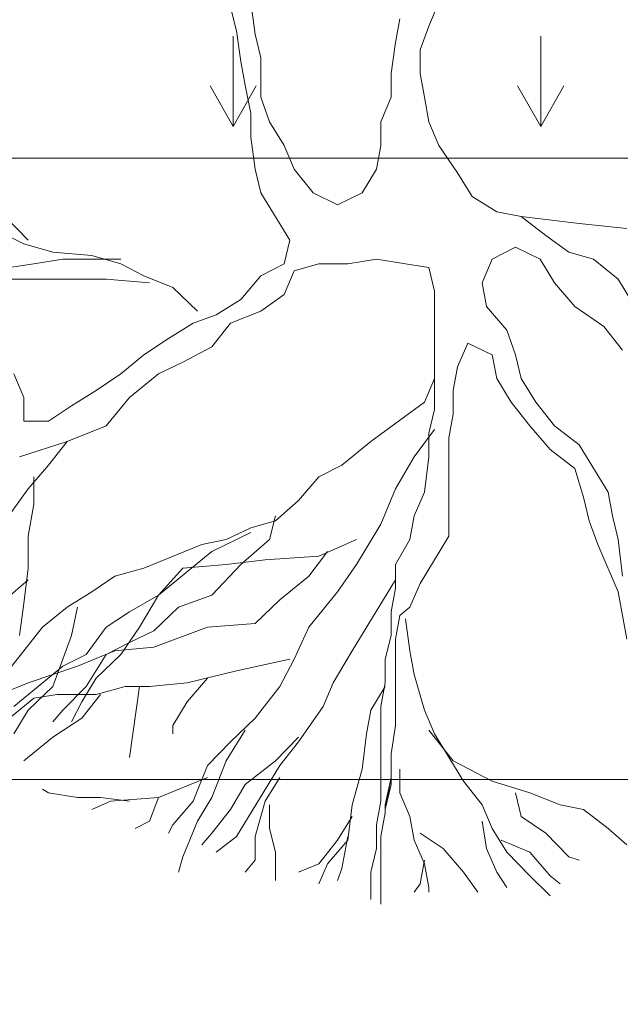
# Model space of a CAD drawing. Units: millimetres. Extents: x 595116 to 630915, y 909473 to 920225.
# Tile 17 of 134: x 629559 to 629582, y 919152 to 919190. Entities that reach past the tile are written whole.
import ezdxf

# ---------------------------------------------------------------- set-up
doc = ezdxf.new("R2010")
doc.units = ezdxf.units.MM
doc.layers.add('Dimension', color=3, linetype='Continuous', lineweight=18)
doc.layers.add('L-PLNT', color=85, linetype='Continuous', lineweight=13)
doc.styles.get("Standard").update_dxf_attribs({"font": 'arial.ttf'})
doc.dimstyles.new('ISO-25', dxfattribs={"dimtxt": 9, "dimasz": 6, "dimexe": 1.25, "dimexo": 0.625, "dimtad": 1, "dimlunit": 4, "dimtxsty": 'Standard', "dimcen": 2.5, "dimadec": 0, "dimazin": 0, "dimtfac": 1, "dimtmove": 0, "dimatfit": 3, "dimfxl": 1, "dimarcsym": 0})

# ---------------------------------------------------------------- blocks, each defined once
blk = doc.blocks.new('A$C143125F4')
for p, q in [((1.7889, 3.3061), (1.767, 3.3957)), ((1.8436, 3.4136), (1.86, 3.2927)), ((2.5164, 3.3241), (2.5547, 3.4136)), ((2.3906, 3.2613), (2.407, 3.3509)), ((2.4836, 3.2345), (2.5164, 3.3241)), ((1.8053, 3.1897), (1.7889, 3.3061)), ((1.86, 3.2927), (1.8819, 3.2031)), ((2.3742, 3.1449), (2.3906, 3.2613)), ((2.4836, 3.1449), (2.4836, 3.2345)), ((1.8217, 3.1001), (1.8053, 3.1897)), ((1.8819, 3.2031), (1.8819, 3.0553)), ((2.3742, 3.0553), (2.3742, 3.1449)), ((2.5, 3.0553), (2.4836, 3.1449)), ((1.8436, 2.9925), (1.8217, 3.1001)), ((1.8819, 3.0553), (1.9147, 2.9612)), ((2.3359, 2.9612), (2.3742, 3.0553)), ((2.5164, 2.9612), (2.5, 3.0553)), ((1.8436, 2.9029), (1.8436, 2.9925)), ((1.9147, 2.9612), (1.9694, 2.8716)), ((2.3359, 2.8716), (2.3359, 2.9612)), ((2.5547, 2.8716), (2.5164, 2.9612)), ((1.86, 2.782), (1.8436, 2.9029)), ((1.9694, 2.8716), (2.0077, 2.782)), ((2.3195, 2.782), (2.3359, 2.8716)), ((2.6259, 2.7686), (2.5547, 2.8716)), ((1.8819, 2.6924), (1.86, 2.782)), ((2.0077, 2.782), (2.0788, 2.6924)), ((2.2648, 2.6924), (2.3195, 2.782)), ((2.6806, 2.679), (2.6259, 2.7686)), ((1.9913, 2.5132), (1.8819, 2.6924)), ((2.0788, 2.6924), (2.1718, 2.6476)), ((2.1718, 2.6476), (2.2648, 2.6924)), ((2.7736, 2.6207), (2.6806, 2.679)), ((2.8666, 2.6028), (2.7736, 2.6207)), ((1.0011, 2.5132), (0.9136, 2.6028)), ((2.8666, 2.6028), (3.0854, 2.5759)), ((2.9596, 2.5311), (2.8666, 2.6028)), ((3.0854, 2.5759), (3.2659, 2.558)), ((0.9847, 2.4998), (0.8917, 2.5446)), ((1.0941, 2.4684), (0.9847, 2.4998)), ((1.9694, 2.4236), (1.9913, 2.5132)), ((3.0471, 2.4684), (2.9596, 2.5311)), ((1.2418, 2.455), (1.0941, 2.4684)), ((2.8447, 2.4863), (2.7571, 2.4415)), ((2.9377, 2.4415), (2.8447, 2.4863)), ((3.1401, 2.4415), (3.0471, 2.4684)), ((1.023, 2.4236), (0.93, 2.4102)), ((1.1324, 2.4415), (1.023, 2.4236)), ((1.3512, 2.4415), (1.1324, 2.4415)), ((1.3512, 2.4236), (1.2418, 2.455)), ((1.4387, 2.3788), (1.3512, 2.4236)), ((1.8819, 2.3788), (1.9694, 2.4236)), ((2.1007, 2.4236), (2.0077, 2.3967)), ((2.2101, 2.4236), (2.1007, 2.4236)), ((2.3195, 2.4415), (2.2101, 2.4236)), ((2.4289, 2.4236), (2.3195, 2.4415)), ((2.5164, 2.4102), (2.4289, 2.4236)), ((2.7571, 2.4415), (2.7189, 2.3519)), ((2.9924, 2.3519), (2.9377, 2.4415)), ((3.2331, 2.3654), (3.1401, 2.4415)), ((2.0077, 2.3967), (1.9694, 2.3071)), ((2.5383, 2.3206), (2.5164, 2.4102)), ((1.2965, 2.3654), (0.93, 2.3654)), ((1.4606, 2.3519), (1.2965, 2.3654)), ((1.5482, 2.334), (1.4387, 2.3788)), ((1.8053, 2.2892), (1.8819, 2.3788)), ((2.7189, 2.3519), (2.7353, 2.2623)), ((3.069, 2.2623), (2.9924, 2.3519)), ((3.2878, 2.2758), (3.2331, 2.3654)), ((1.6412, 2.2444), (1.5482, 2.334)), ((2.5383, 1.8726), (2.5383, 2.3206)), ((1.7123, 2.231), (1.8053, 2.2892)), ((1.9694, 2.3071), (1.8819, 2.2444)), ((1.8819, 2.2444), (1.767, 2.1996)), ((2.7353, 2.2623), (2.8119, 2.1727)), ((3.1784, 2.1862), (3.069, 2.2623)), ((1.5317, 2.1414), (1.6247, 2.1996)), ((1.6247, 2.1996), (1.7123, 2.231)), ((1.767, 2.1996), (1.6959, 2.11)), ((2.8119, 2.1727), (2.8447, 2.0787)), ((3.2495, 2.0966), (3.1784, 2.1862)), ((1.4387, 2.0787), (1.5317, 2.1414)), ((1.6959, 2.11), (1.5865, 2.0518)), ((2.6641, 2.1235), (2.6259, 2.0339)), ((2.7571, 2.0787), (2.6641, 2.1235)), ((1.3512, 2.007), (1.4387, 2.0787)), ((1.5865, 2.0518), (1.4935, 2.007)), ((2.7736, 1.9891), (2.7571, 2.0787)), ((2.8447, 2.0787), (2.8666, 1.9891)), ((2.6259, 2.0339), (2.6094, 1.9443)), ((0.9464, 2.007), (0.9847, 1.9174)), ((1.2582, 1.9443), (1.3512, 2.007)), ((1.4935, 2.007), (1.384, 1.9174)), ((2.5383, 1.9891), (2.5, 1.8995)), ((2.8283, 1.8995), (2.7736, 1.9891)), ((2.8666, 1.9891), (2.9213, 1.8995)), ((1.1652, 1.886), (1.2582, 1.9443)), ((2.6094, 1.9443), (2.6094, 1.8547)), ((0.9847, 1.9174), (0.9847, 1.8278)), ((1.384, 1.9174), (1.2965, 1.8099)), ((1.0777, 1.8278), (1.1652, 1.886)), ((2.5, 1.8995), (2.2976, 1.7516)), ((2.5164, 1.783), (2.5383, 1.8726)), ((2.8994, 1.8099), (2.8283, 1.8995)), ((2.9213, 1.8995), (2.9924, 1.8099)), ((0.9847, 1.8278), (1.0777, 1.8278)), ((2.6094, 1.8547), (2.593, 1.7651)), ((1.2965, 1.8099), (1.1488, 1.7516)), ((2.5383, 1.7964), (2.4617, 1.6934)), ((2.976, 1.7203), (2.8994, 1.8099)), ((2.9924, 1.8099), (3.0854, 1.7382)), ((2.5164, 1.6934), (2.5164, 1.783)), ((2.593, 1.7651), (2.593, 1.3932)), ((1.1488, 1.7516), (0.9683, 1.6934)), ((1.1488, 1.7516), (1.0777, 1.662)), ((2.2976, 1.7516), (2.1882, 1.662)), ((3.069, 1.6486), (2.976, 1.7203)), ((3.0854, 1.7382), (3.1948, 1.559)), ((2.4617, 1.6934), (2.3906, 1.5724)), ((2.5, 1.559), (2.5164, 1.6934)), ((1.0777, 1.662), (1.0011, 1.5724)), ((2.1882, 1.662), (2.1007, 1.6172)), ((3.1018, 1.5411), (3.069, 1.6486)), ((1.023, 1.6172), (1.023, 1.5142)), ((2.1007, 1.6172), (2.0241, 1.5276)), ((1.0011, 1.5724), (0.9136, 1.4515)), ((2.3906, 1.5724), (2.3359, 1.438)), ((2.4617, 1.4694), (2.5, 1.559)), ((3.1237, 1.4515), (3.1018, 1.5411)), ((3.1948, 1.559), (3.2112, 1.4694)), ((1.023, 1.5142), (1.0011, 1.3932)), ((2.0241, 1.5276), (1.9366, 1.4515)), ((1.9366, 1.4694), (1.9147, 1.3798)), ((2.4453, 1.3798), (2.4617, 1.4694)), ((3.2112, 1.4694), (3.2331, 1.3798)), ((1.8436, 1.4246), (1.7506, 1.3798)), ((1.9366, 1.4515), (1.8436, 1.4246)), ((2.3359, 1.438), (2.2429, 1.2857)), ((3.1565, 1.3619), (3.1237, 1.4515)), ((1.0011, 1.3932), (1.0011, 1.2723)), ((1.7506, 1.3798), (1.6576, 1.3619)), ((1.8436, 1.4067), (1.6959, 1.335)), ((1.9147, 1.3798), (1.8053, 1.2857)), ((2.2429, 1.3798), (2.1007, 1.3171)), ((2.3906, 1.2857), (2.4453, 1.3798)), ((2.593, 1.3932), (2.4836, 1.214)), ((3.2331, 1.3798), (3.2495, 1.2409)), ((1.6576, 1.3619), (1.4387, 1.2723)), ((3.2331, 1.1827), (3.1565, 1.3619)), ((1.6959, 1.335), (1.4935, 1.1692)), ((2.1007, 1.3171), (1.8983, 1.3036)), ((2.1335, 1.335), (2.0624, 1.2409)), ((1.0011, 1.2723), (0.9847, 1.1379)), ((1.4387, 1.2723), (1.3293, 1.2409)), ((1.5865, 1.2723), (1.4935, 1.1692)), ((1.7506, 1.2857), (1.5865, 1.2723)), ((1.8053, 1.2857), (1.6959, 1.1692)), ((1.8983, 1.3036), (1.7506, 1.2857)), ((2.2429, 1.2857), (2.1718, 1.1827)), ((2.3906, 1.1961), (2.3906, 1.2857)), ((1.3293, 1.2409), (1.2418, 1.1827)), ((2.0624, 1.2409), (1.953, 1.1513)), ((1.0011, 1.2275), (0.9136, 1.1513)), ((2.3906, 1.2275), (2.2265, 0.9587)), ((2.3742, 1.1065), (2.3906, 1.1961)), ((2.4836, 1.214), (2.4453, 1.1244)), ((1.2418, 1.1827), (1.1488, 1.1244)), ((1.4935, 1.1692), (1.384, 1.1065)), ((1.4935, 1.1692), (1.4223, 1.0483)), ((1.6959, 1.1692), (1.57, 1.1244)), ((2.1718, 1.1827), (2.0624, 1.0483)), ((3.2659, 1.0035), (3.2331, 1.1827)), ((0.9847, 1.1379), (0.9683, 1.0169)), ((1.1488, 1.1244), (1.0558, 1.0483)), ((1.1871, 1.1244), (1.1652, 1.0169)), ((1.57, 1.1244), (1.477, 1.0348)), ((1.953, 1.1513), (1.86, 1.0617)), ((2.4453, 1.1244), (2.407, 1.0931)), ((1.384, 1.1065), (1.2965, 1.0483)), ((2.3742, 1.0169), (2.3742, 1.1065)), ((2.407, 1.0931), (2.3906, 1.0035)), ((1.0558, 1.0483), (0.9136, 0.8691)), ((1.2965, 1.0483), (1.2199, 0.9452)), ((1.4223, 1.0483), (1.3512, 0.9452)), ((1.6795, 1.0483), (1.477, 0.9721)), ((1.86, 1.0617), (1.6795, 1.0483)), ((2.0624, 1.0483), (2.0077, 0.9273)), ((2.4289, 1.0796), (2.4453, 0.9587)), ((1.1652, 1.0169), (1.1324, 0.9273)), ((1.477, 1.0348), (1.384, 0.99)), ((2.3523, 0.9273), (2.3742, 1.0169)), ((1.384, 0.99), (1.2965, 0.9452)), ((1.477, 0.9721), (1.3293, 0.9587)), ((2.3906, 1.0035), (2.3906, 0.6765)), ((1.2199, 0.9452), (1.1324, 0.9005)), ((1.3293, 0.9587), (1.1871, 0.9005)), ((1.2965, 0.9452), (1.2199, 0.8243)), ((1.3512, 0.9452), (1.2582, 0.8557)), ((2.2265, 0.9587), (2.1554, 0.8377)), ((2.4453, 0.9587), (2.4617, 0.8691)), ((1.1324, 0.9005), (0.9464, 0.7481)), ((1.1871, 0.9005), (1.0011, 0.8377)), ((1.1324, 0.9273), (1.0941, 0.8243)), ((1.9913, 0.9273), (1.7889, 0.8825)), ((2.0077, 0.9273), (1.953, 0.8243)), ((2.3523, 0.8377), (2.3523, 0.9273)), ((1.7889, 0.8825), (1.6029, 0.8377)), ((2.4617, 0.8691), (2.5, 0.7347)), ((1.0011, 0.8377), (0.7823, 0.7481)), ((1.0941, 0.8243), (1.0011, 0.7347)), ((1.2199, 0.8243), (1.1324, 0.7347)), ((1.2582, 0.8557), (1.2035, 0.7661)), ((1.3676, 0.8243), (1.2582, 0.7929)), ((1.4606, 0.8243), (1.3676, 0.8243)), ((1.4223, 0.8243), (1.384, 0.5555)), ((1.6029, 0.8377), (1.4606, 0.8243)), ((1.6795, 0.8557), (1.6029, 0.7661)), ((1.953, 0.8243), (1.86, 0.7033)), ((2.1554, 0.8377), (2.1171, 0.7481)), ((2.3523, 0.8243), (2.2976, 0.7347)), ((2.3359, 0.7481), (2.3523, 0.8377)), ((1.1105, 0.7929), (1.023, 0.7795)), ((1.2582, 0.7929), (1.1105, 0.7929)), ((1.2746, 0.7929), (1.2035, 0.7033)), ((1.023, 0.7795), (0.93, 0.7033)), ((1.2035, 0.7661), (1.1652, 0.6899)), ((1.6029, 0.7661), (1.5482, 0.6765)), ((2.1171, 0.7481), (2.0241, 0.6137)), ((2.3359, 0.3897), (2.3359, 0.7481)), ((1.0011, 0.7347), (0.9464, 0.6451)), ((1.1324, 0.7347), (1.0941, 0.6899)), ((2.2976, 0.7347), (2.2812, 0.6451)), ((2.5, 0.7347), (2.5383, 0.6451)), ((1.2035, 0.7033), (1.0941, 0.6317)), ((1.5482, 0.6765), (1.5482, 0.6451)), ((1.86, 0.7033), (1.767, 0.6137)), ((2.3906, 0.6765), (2.3742, 0.5689)), ((1.8217, 0.6585), (1.7506, 0.5421)), ((2.2812, 0.6451), (2.2648, 0.5107)), ((2.5164, 0.6585), (2.6094, 0.5421)), ((2.5383, 0.6451), (2.6477, 0.4659)), ((1.0941, 0.6317), (0.9847, 0.5421)), ((1.767, 0.6137), (1.6795, 0.5241)), ((2.0241, 0.6317), (1.9366, 0.5421)), ((2.0241, 0.6137), (1.953, 0.5241)), ((2.3742, 0.5689), (2.3742, 0.4525)), ((1.6795, 0.5241), (1.6247, 0.3897)), ((1.7506, 0.5421), (1.6959, 0.4032)), ((1.953, 0.5241), (1.7889, 0.2554)), ((1.9366, 0.5421), (1.8217, 0.4525)), ((2.6094, 0.5421), (2.7571, 0.4659)), ((2.2648, 0.5107), (2.2265, 0.3763)), ((2.407, 0.5107), (2.407, 0.4211)), ((1.6795, 0.4793), (1.4935, 0.4032)), ((1.8217, 0.4525), (1.767, 0.3584)), ((1.953, 0.4793), (1.8983, 0.3897)), ((2.3523, 0.3584), (2.3742, 0.4793)), ((2.3742, 0.4793), (2.3523, 0.3763)), ((2.3742, 0.4525), (2.3523, 0.3584)), ((2.6477, 0.4659), (2.7189, 0.3763)), ((2.7571, 0.4659), (2.8994, 0.4211)), ((1.0777, 0.4211), (1.0558, 0.4345)), ((1.1871, 0.4032), (1.0777, 0.4211)), ((2.407, 0.4211), (2.4453, 0.3315)), ((2.8447, 0.4211), (2.8666, 0.3315)), ((2.8994, 0.4211), (3.0143, 0.3763)), ((1.2746, 0.4032), (1.1871, 0.4032)), ((1.3129, 0.3897), (1.2418, 0.3584)), ((1.384, 0.3897), (1.2746, 0.4032)), ((1.4935, 0.4032), (1.3129, 0.3897)), ((1.4935, 0.4032), (1.4606, 0.3136)), ((1.6247, 0.3897), (1.5482, 0.3002)), ((1.6959, 0.4032), (1.6412, 0.3136)), ((1.8983, 0.3897), (1.86, 0.2554)), ((1.9147, 0.3763), (1.9147, 0.2867)), ((2.2265, 0.3763), (2.2101, 0.2419)), ((2.3195, 0.3002), (2.3359, 0.3897)), ((2.3523, 0.3763), (2.3523, 0.3449)), ((2.7189, 0.3763), (2.7571, 0.2867)), ((3.0143, 0.3763), (3.1018, 0.3584)), ((1.767, 0.3584), (1.6959, 0.2688)), ((2.3523, 0.3449), (2.3359, 0.2554)), ((3.1018, 0.3584), (3.1948, 0.2867)), ((1.4606, 0.3136), (1.4059, 0.2867)), ((1.5482, 0.3002), (1.5317, 0.2688)), ((1.6412, 0.3136), (1.5865, 0.1792)), ((2.2265, 0.3315), (2.1718, 0.2419)), ((2.3195, 0.2106), (2.3195, 0.3002)), ((2.4453, 0.3315), (2.4617, 0.2419)), ((2.7189, 0.3136), (2.7353, 0.2106)), ((2.8666, 0.3315), (2.9596, 0.2688)), ((1.6959, 0.2688), (1.6576, 0.224)), ((1.9147, 0.2867), (1.9366, 0.1971)), ((2.4836, 0.2688), (2.5711, 0.2106)), ((2.7571, 0.2867), (2.8119, 0.1971)), ((2.9596, 0.2688), (3.0471, 0.1792)), ((3.1948, 0.2867), (3.2659, 0.224)), ((1.7889, 0.2554), (1.7123, 0.1971)), ((1.86, 0.2554), (1.86, 0.1658)), ((2.1718, 0.2419), (2.1007, 0.1523)), ((2.2101, 0.2419), (2.1335, 0.1523)), ((2.2101, 0.2554), (2.1882, 0.1344)), ((2.3359, 0.2554), (2.3359, 0)), ((2.4617, 0.2419), (2.5, 0.1523)), ((2.79, 0.2419), (2.8994, 0.1971)), ((1.9366, 0.1971), (1.9366, 0.0896)), ((2.2976, 0.121), (2.3195, 0.2106)), ((2.5711, 0.2106), (2.6477, 0.121)), ((2.7353, 0.2106), (2.7736, 0.121)), ((2.8119, 0.1971), (2.8994, 0.1075)), ((2.8994, 0.1971), (2.976, 0.1075)), ((1.5865, 0.1792), (1.57, 0.121)), ((1.86, 0.1658), (1.8217, 0.121)), ((2.1007, 0.1523), (2.0241, 0.121)), ((2.1335, 0.1523), (2.1007, 0.0762)), ((2.5, 0.1658), (2.4836, 0.0762)), ((2.5, 0.1523), (2.5164, 0.0627)), ((3.0471, 0.1792), (3.0854, 0.1658)), ((2.1882, 0.1344), (2.1718, 0.0896)), ((2.2976, 0.0179), (2.2976, 0.121)), ((2.6477, 0.121), (2.7024, 0.0448)), ((2.7736, 0.121), (2.8119, 0.0627)), ((2.4836, 0.0762), (2.4617, 0.0448)), ((2.8994, 0.1075), (2.976, 0.0314)), ((2.976, 0.1075), (3.0143, 0.0762)), ((2.5164, 0.0627), (2.5164, 0.0448))]:
    blk.add_line(p, q)
blk = doc.blocks.new('LAWN-GRASS-TUFT')
blk.add_line((0.892, 3.485), (0.892, 0))
blk.add_lwpolyline([(0, 1.577), (0.892, 0), (1.785, 1.577)])
blk = doc.blocks.new('*D216')
at = {"layer": 'Defpoints', "color": 0, "transparency": 16777216}
for p in [(629505.041, 919411.828), (629743.541, 919411.928), (629743.541, 918832.378)]:
    blk.add_point(p, dxfattribs=at)
at = {"layer": 'Dimension', "color": 0, "lineweight": -2, "transparency": 16777216}
for p, q in [((629505.041, 919411.203), (629505.041, 918831.128)), ((629743.541, 919411.303), (629743.541, 918831.128)), ((629511.041, 918832.378), (629737.541, 918832.378))]:
    blk.add_line(p, q, dxfattribs=at)
at = {"layer": 'Dimension', "color": 0, "transparency": 16777216}
for points in [[(629511.041, 918833.378), (629511.041, 918831.378), (629505.041, 918832.378)], [(629737.541, 918833.378), (629737.541, 918831.378), (629743.541, 918832.378)]]:
    blk.add_solid(points, dxfattribs=at)
at = {"layer": 'Dimension', "color": 0, "transparency": 16777216, "insert": (629624.291, 918837.656), "char_height": 9, "attachment_point": 5}
blk.add_mtext('19\'-10 1/2"', dxfattribs=at)

msp = doc.modelspace()

# ---------------------------------------------------------------- linework, layer by layer
at = {"layer": 'L-PLNT'}
for p, q in [((629535.274, 919184.917), (629800.951, 919184.917)), ((629511.274, 919160.917), (629824.951, 919160.917))]:
    msp.add_line(p, q, dxfattribs=at)

# ---------------------------------------------------------------- block references
at = {"layer": 'L-PLNT', "xscale": 10.20167662382051, "yscale": 10.20167662382051, "zscale": 10.20167662382051}
msp.add_blockref('A$C143125F4', (629549.214, 919156.111), dxfattribs=at)
at = {"layer": 'L-PLNT'}
for p in [(629566.446, 919186.14), (629578.319, 919186.14)]:
    msp.add_blockref('LAWN-GRASS-TUFT', p, dxfattribs=at)

# ---------------------------------------------------------------- dimensions: what is measured, and where the dimension line sits
at = {"layer": 'Dimension'}
dim = msp.add_linear_dim(base=(629743.541, 918832.378), p1=(629505.041, 919411.828), p2=(629743.541, 919411.928), dimstyle='ISO-25', override={"dimdec": 1, "dimlfac": 1, "dimrnd": 0, "dimzin": 1, "dimdsep": 46, "dimlunit": 4, "dimfrac": 2}, dxfattribs=at)
dim.commit()
dim.dimension.update_dxf_attribs({"geometry": '*D216', "text_midpoint": (629624.291, 918837.656)})

doc.saveas('drawing.dxf')
